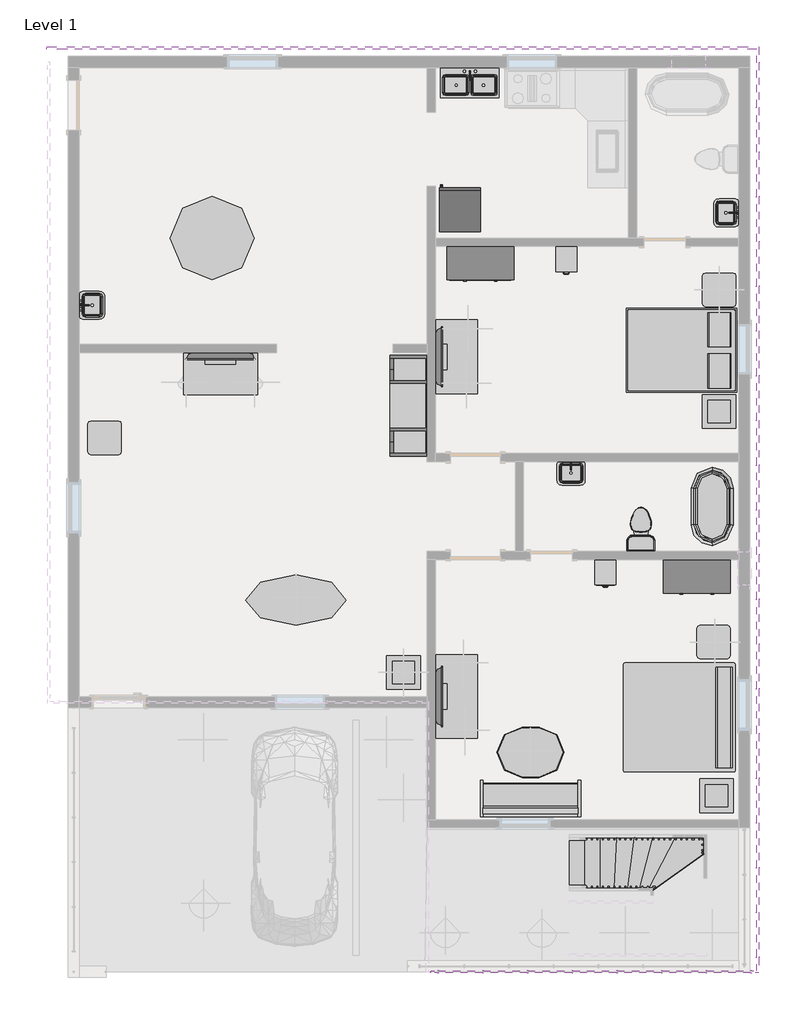
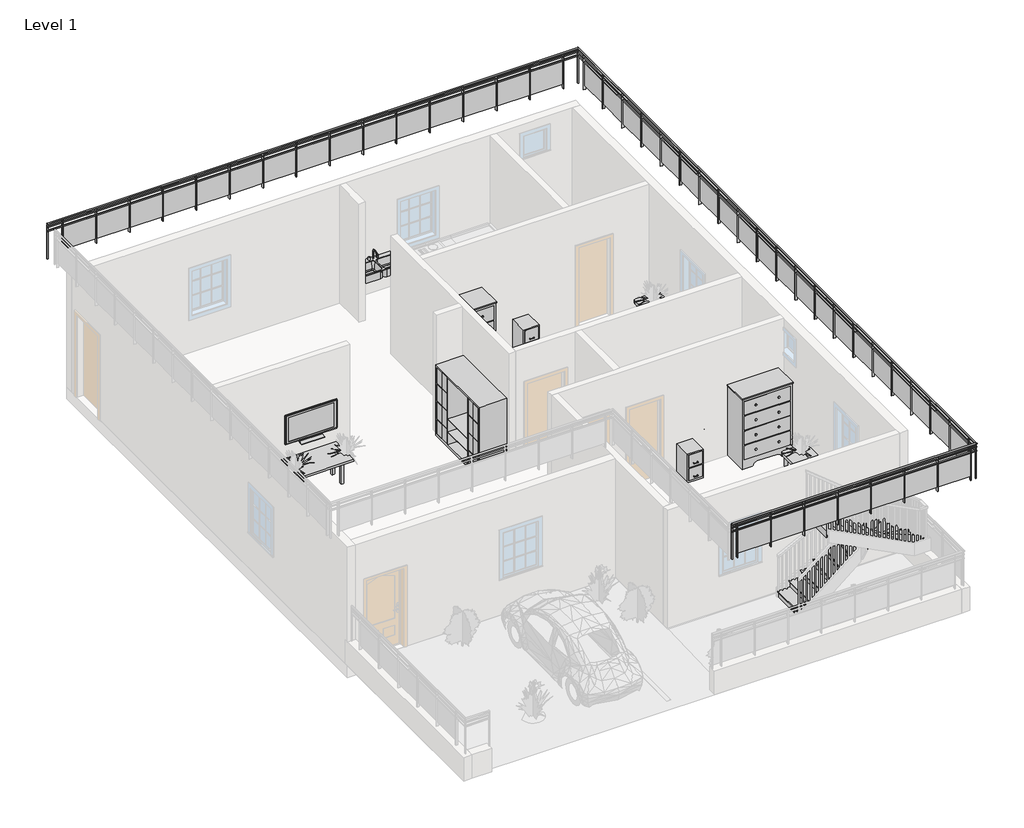
# One storey, part 4 of 5: 23 furniture elements, 7 flow terminals, 1 proxy, 1 railing, 1 stair flight.
# Revit data of these elements (continued)
# Element 6 (IfcFlowTerminal, "Sink Vanity-Square : 20\" x 18\"")
#   Mark = "7"
#   Phase Created = New Construction
#   Materials on its faces: "Porcelain, Linen", "Steel, Polished"
# Element 7 (IfcFlowTerminal, "Toilet-Domestic-3D : Toilet-Domestic-3D")
#   Mark = "9"
#   Phase Created = New Construction
#   Materials on its faces: "Porcelain, Linen", "Laminate, Linen, Matte"
# Element 8 (IfcFlowTerminal, "Tub-Free Standing-3D : 30\" x 60\" 2")
#   Mark = "8"
#   Phase Created = New Construction
#   Materials on its faces: "Porcelain, Ivory"
# Element 9 (IfcFurniture, "Bed-Box : Queen 60\" x 79\"")
#   Phase Created = New Construction
#   Materials on its faces: "Birch", "Oak Flooring"
# Element 10 (IfcFurniture, "Bed-Standard.0001 : King 78\" x 80\"")
#   Phase Created = New Construction
#   Materials on its faces: "Linen, White", "Steel, Chrome Plated"
# Elements 11, 12 (IfcFurniture, "Cabinet-File 2 Drawer : 15\" x 18\"")
#   Phase Created = New Construction
#   Materials on its faces: "Steel, Chrome Plated", "Steel, Paint Finish, Ivory, Glossy"
# Elements 13, 14 (IfcFurniture, "Dresser : 48\" x 72\" x 24\"")
#   Phase Created = New Construction
#   Materials on its faces: "Laminate, Ivory, Matte", "Cherry", "Wood - Teak"
# Element 15 (IfcFurniture, "Entertainment Center : 72\" x 72\" x 24\"")
#   Phase Created = New Construction
#   Materials on its faces: "Porcelain, Linen", "Steel, Chrome Plated", "Glass - Clear, Grey"
# Element 16 (IfcFurniture, "Sofa : 72\"")
#   Phase Created = New Construction
#   Materials on its faces: "Cherry", "Linen, Beige"
# Elements 17, 18 (IfcFurniture, "TV - Flat Screen : 42\"")
#   Stand = yes
#   Phase Created = New Construction
#   Materials on its faces: "TV - Black", "TV - Glass", "TV - Screen"
# Element 19 (IfcFurniture, "TV - Flat Screen : 50\"")
#   Stand = yes
#   Phase Created = New Construction
#   Materials on its faces: "TV - Black", "TV - Glass", "TV - Screen"
# Elements 20, 21, 22 (IfcFurniture, "Table-Coffee : 24\" x 24\" x 24\"")
#   Phase Created = New Construction
#   Materials on its faces: "Glass - Clear, Grey"
# Element 23 (IfcFurniture, "Table-Dining Oval : 36\" x 48\"")
#   Phase Created = New Construction
#   Materials on its faces: "Steel, Chrome Plated", "Glass - Clear, Grey"
# Element 24 (IfcFurniture, "Table-Dining Round w Chairs : 60\" Diameter")
#   Phase Created = New Construction
#   Materials on its faces: "Pine", "Laminate, Linen, Matte"
# Element 25 (IfcFurniture, "Table-Ellipse : 72\" x 36\"")
#   Phase Created = New Construction
#   Materials on its faces: "Birch", "Plywood, Sheathing"
# Elements 26, 27, 28 (IfcFurniture, "Table-End : 24\" x 24\"")
#   Phase Created = New Construction
#   Materials on its faces: "Laminate, Ivory, Matte", "Birch"
# Elements 29, 30 (IfcFurniture, "Table-Rectangular : 72\" x 30\"")
#   Phase Created = New Construction
#   Materials on its faces: "Birch"
# Element 31 (IfcFurniture, "Table-Rectangular : 72\" x 30\" 2")
#   Phase Created = New Construction
#   Materials on its faces: "Birch"
# Element 32 (IfcRailing, "Glass Panel - Bottom Fill")
#   built-in parameter 1008621 = 11 (stored number, unit not read)
#   Phase Created = New Construction
#   Materials on its faces: "Glass"
# Element 33 (IfcStairFlight, "2\" Tread 1\" Nosing 1/4\" Riser")
#   Phase Created = New Construction
# Materials
#   "Cherry": class "Wood", colour RGB 226 177 128, transparency 0, Description = "Prunus Serotina", Cost = 0
#   "Steel, Polished": class "Metal", colour RGB 57 57 57, transparency 0, Description = "Polished steel", Cost = 0
#   "Porcelain, Linen": class "Ceramic", colour RGB 249 239 230, transparency 0, Description = "Porcelain, linen", Cost = 0
#   "Laminate, Linen, Matte": class "Plastic", colour RGB 249 239 230, transparency 0, Description = "Plastic Laminate - Linen, Matte", Cost = 0
#   "Porcelain, Ivory": class "Ceramic", colour RGB 247 247 239, transparency 0, Description = "Porcelain, ivory", Cost = 0
#   "Birch": class "Wood", colour RGB 210 159 95, transparency 0, Description = "Betula Alleghaniensis", Cost = 0
#   "Oak Flooring": class "Wood", colour RGB 216 169 114, transparency 0, Description = "Quercus Rubra", Cost = 0
#   "Steel, Chrome Plated": class "Metal", colour RGB 17 17 17, transparency 0, Description = "Chromiuim plated steel", Cost = 0
#   "Linen, Beige": class "Textile", colour RGB 249 239 230, transparency 0, Description = "Linen, beige", Cost = 0
#   "Steel, Paint Finish, Ivory, Glossy": class "Metal", colour RGB 247 247 239, transparency 0, Description = "Steel, paint finish, ivory, glossy", Cost = 0
#   "Wood - Teak": class "Wood", colour RGB 145 112 90, transparency 0
#   "Glass - Clear, Grey": class "Glass", colour RGB 252 255 255, transparency 0.64
#   "Pine": class "Wood", colour RGB 223 192 134, transparency 0, Description = "Pinus Echinata", Cost = 0
#   "Plywood, Sheathing": class "Wood", colour RGB 212 179 113, transparency 0, Description = "Plywood, sheathing grade", Cost = 0
#   "Laminate, Ivory, Matte": class "Plastic", colour RGB 247 247 239, transparency 0, Description = "Plastic Laminate - Ivory, Matte", Cost = 0
#   "Linen, White": class "Textile", colour RGB 247 247 239, transparency 0, Description = "Linen, white", Cost = 0
#   "TV - Black": colour RGB 49 49 49, transparency 0
#   "TV - Glass": colour RGB 157 157 157, transparency 0.9
#   "TV - Screen": colour RGB 0 0 0, transparency 0
#   "Glass": class "Glass", colour RGB 0 128 192, transparency 0.75, Description = "Soda Lime Glass", Cost = 0
